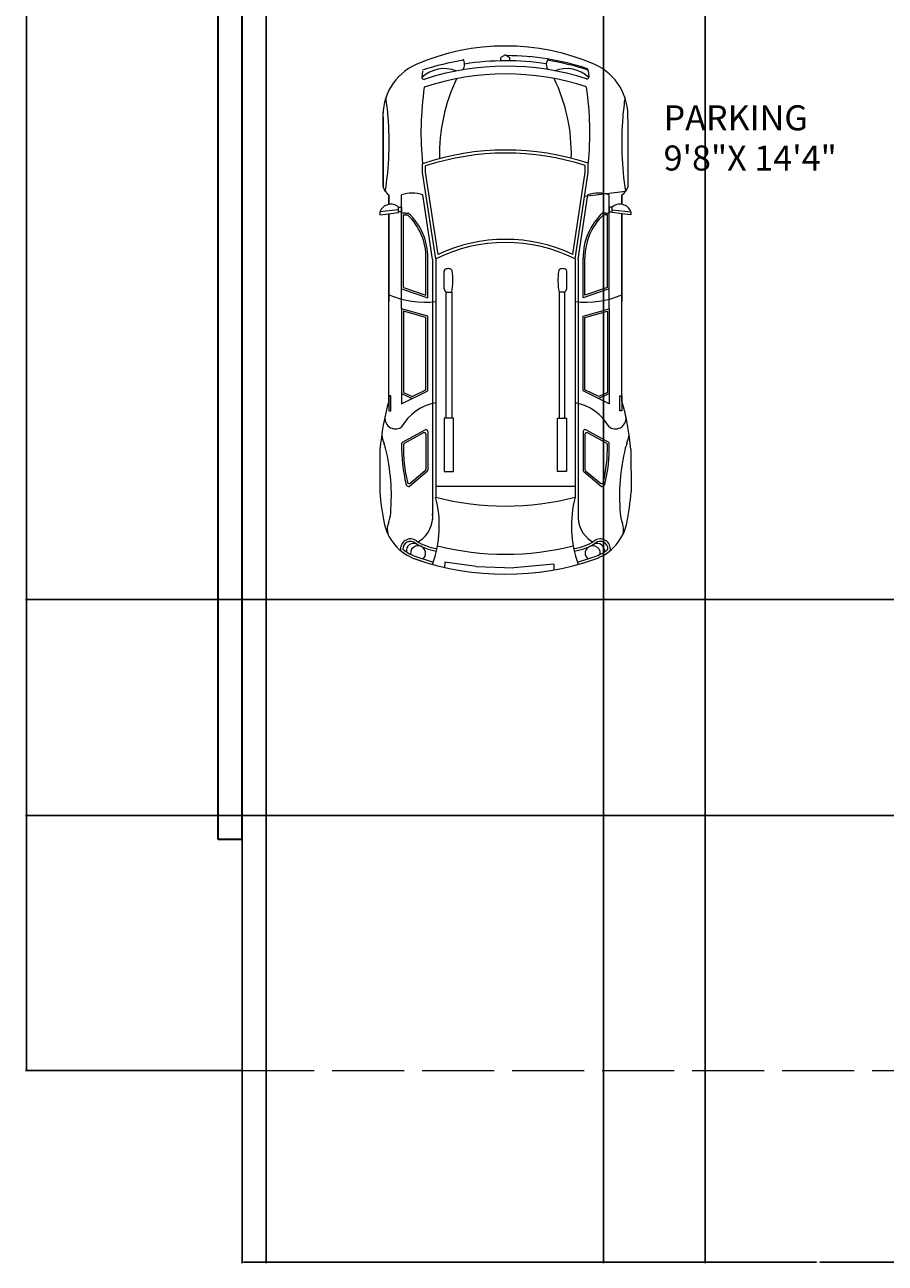
# Model space of a CAD drawing. Units: feet. Extents: x 1993 to 2298, y 2938 to 3641.
# Tile 1 of 11: x 1993 to 2137, y 2938 to 3144. Entities that reach past the tile are written whole.
import ezdxf

# ---------------------------------------------------------------- set-up
doc = ezdxf.new("R2010")
doc.units = ezdxf.units.FT
doc.linetypes.add('ACAD_ISO02W100', pattern=[15, 12, -3])
for name, color, linetype, lineweight in [('A-ANNO-DIMS', 2, 'Continuous', 18), ('A-AREA-IDEN', 7, 'Continuous', 18), ('A-EQPM-VEHC', 8, 'Continuous', 13), ('SUNSHADES', 4, 'ACAD_ISO02W100', 13), ('WAL', 7, 'Continuous', 35)]:
    doc.layers.add(name, color=color, linetype=linetype, lineweight=lineweight)
doc.styles.get("Standard").update_dxf_attribs({"font": 'arial.ttf'})
doc.dimstyles.get("Standard").update_dxf_attribs({"dimtxt": 0.18, "dimasz": 0.18, "dimexe": 0.18, "dimexo": 0.0625, "dimgap": 0.09, "dimtad": 0, "dimtih": 1, "dimtoh": 1, "dimdec": 4, "dimzin": 0, "dimdsep": 46, "dimtxsty": 'Standard', "dimcen": 0.09, "dimadec": 0, "dimazin": 0, "dimtfac": 1, "dimtdec": 4, "dimtofl": 0, "dimtmove": 0, "dimatfit": 3, "dimfxl": 1, "dimtolj": 1, "dimtzin": 0, "dimarcsym": 0})

# ---------------------------------------------------------------- blocks, each defined once
blk = doc.blocks.new('*D56')
at = {"layer": 'A-ANNO-DIMS', "color": 0, "lineweight": -2, "transparency": 16777216}
for p, q in [((2025.7, 3608.53), (1993.61, 3608.53)), ((1993.79, 3608.35), (1993.79, 3289.45)), ((1993.79, 2970.18), (1993.79, 3289.08)), ((2029.7, 2970), (1993.61, 2970))]:
    blk.add_line(p, q, dxfattribs=at)
at = {"layer": 'A-ANNO-DIMS', "color": 0, "transparency": 16777216}
for points in [[(1993.76, 3608.35), (1993.82, 3608.35), (1993.79, 3608.53)], [(1993.76, 2970.18), (1993.82, 2970.18), (1993.79, 2970)]]:
    blk.add_solid(points, dxfattribs=at)
at = {"layer": 'Defpoints', "color": 0, "transparency": 16777216}
for p in [(1993.79, 3608.53), (2025.76, 3608.53), (2029.76, 2970)]:
    blk.add_point(p, dxfattribs=at)
at = {"layer": 'A-ANNO-DIMS', "color": 0, "transparency": 16777216, "insert": (1993.79, 3289.27), "char_height": 0.18, "attachment_point": 5}
blk.add_mtext('\\A1;638.5', dxfattribs=at)
blk = doc.blocks.new('*D57')
at = {"layer": 'A-ANNO-DIMS', "color": 0, "lineweight": -2, "transparency": 16777216}
for p, q in [((2029.76, 2969.94), (2029.76, 2937.86)), ((2221.76, 2969.94), (2221.76, 2937.86)), ((2029.94, 2938.03), (2125.48, 2938.03)), ((2221.58, 2938.03), (2126.04, 2938.03))]:
    blk.add_line(p, q, dxfattribs=at)
at = {"layer": 'A-ANNO-DIMS', "color": 0, "transparency": 16777216}
for points in [[(2029.94, 2938.07), (2029.94, 2938.01), (2029.76, 2938.03)], [(2221.58, 2938.07), (2221.58, 2938.01), (2221.76, 2938.03)]]:
    blk.add_solid(points, dxfattribs=at)
at = {"layer": 'Defpoints', "color": 0, "transparency": 16777216}
for p in [(2029.76, 2970), (2221.76, 2970), (2221.76, 2938.03)]:
    blk.add_point(p, dxfattribs=at)
at = {"layer": 'A-ANNO-DIMS', "color": 0, "transparency": 16777216, "insert": (2125.76, 2938.03), "char_height": 0.18, "attachment_point": 5}
blk.add_mtext('\\A1;192', dxfattribs=at)
blk = doc.blocks.new('*D58')
at = {"layer": 'A-ANNO-DIMS', "color": 0, "lineweight": -2, "transparency": 16777216}
for p, q in [((2139.94, 3048.53), (1993.61, 3048.53)), ((1993.79, 3048.35), (1993.79, 3030.72)), ((1993.79, 3012.71), (1993.79, 3030.35)), ((2139.94, 3012.53), (1993.61, 3012.53))]:
    blk.add_line(p, q, dxfattribs=at)
at = {"layer": 'A-ANNO-DIMS', "color": 0, "transparency": 16777216}
for points in [[(1993.76, 3048.35), (1993.82, 3048.35), (1993.79, 3048.53)], [(1993.76, 3012.71), (1993.82, 3012.71), (1993.79, 3012.53)]]:
    blk.add_solid(points, dxfattribs=at)
at = {"layer": 'Defpoints', "color": 0, "transparency": 16777216}
for p in [(1993.79, 3048.53), (2140, 3048.53), (2140, 3012.53)]:
    blk.add_point(p, dxfattribs=at)
at = {"layer": 'A-ANNO-DIMS', "color": 0, "transparency": 16777216, "insert": (1993.79, 3030.53), "char_height": 0.18, "attachment_point": 5}
blk.add_mtext('\\A1;36', dxfattribs=at)
blk = doc.blocks.new('*D67')
at = {"layer": 'A-ANNO-DIMS', "color": 0, "lineweight": -2, "transparency": 16777216}
for p, q in [((2033.76, 3428.47), (2033.76, 2937.86)), ((2106.96, 3428.47), (2106.96, 2937.86)), ((2033.94, 2938.03), (2070.03, 2938.03)), ((2106.78, 2938.03), (2070.68, 2938.03))]:
    blk.add_line(p, q, dxfattribs=at)
at = {"layer": 'A-ANNO-DIMS', "color": 0, "transparency": 16777216}
for points in [[(2033.94, 2938.07), (2033.94, 2938.01), (2033.76, 2938.03)], [(2106.78, 2938.07), (2106.78, 2938.01), (2106.96, 2938.03)]]:
    blk.add_solid(points, dxfattribs=at)
at = {"layer": 'Defpoints', "color": 0, "transparency": 16777216}
for p in [(2033.76, 3428.53), (2106.96, 3428.53), (2106.96, 2938.03)]:
    blk.add_point(p, dxfattribs=at)
at = {"layer": 'A-ANNO-DIMS', "color": 0, "transparency": 16777216, "insert": (2070.36, 2938.03), "char_height": 0.18, "attachment_point": 5}
blk.add_mtext('\\A1;73.2', dxfattribs=at)
blk = doc.blocks.new('*D71')
at = {"layer": 'A-ANNO-DIMS', "color": 0, "lineweight": -2, "transparency": 16777216}
for p, q in [((2029.76, 3159.94), (2029.76, 2937.86)), ((2090, 3159.94), (2090, 2937.86)), ((2029.94, 2938.03), (2059.49, 2938.03)), ((2089.82, 2938.03), (2060.27, 2938.03))]:
    blk.add_line(p, q, dxfattribs=at)
at = {"layer": 'A-ANNO-DIMS', "color": 0, "transparency": 16777216}
for points in [[(2029.94, 2938.07), (2029.94, 2938.01), (2029.76, 2938.03)], [(2089.82, 2938.07), (2089.82, 2938.01), (2090, 2938.03)]]:
    blk.add_solid(points, dxfattribs=at)
at = {"layer": 'Defpoints', "color": 0, "transparency": 16777216}
for p in [(2029.76, 3160), (2090, 3160), (2090, 2938.03)]:
    blk.add_point(p, dxfattribs=at)
at = {"layer": 'A-ANNO-DIMS', "color": 0, "transparency": 16777216, "insert": (2059.88, 2938.03), "char_height": 0.18, "attachment_point": 5}
blk.add_mtext('\\A1;60.24', dxfattribs=at)
blk = doc.blocks.new('*D75')
at = {"layer": 'A-ANNO-DIMS', "color": 0, "lineweight": -2, "transparency": 16777216}
for p, q in [((2029.76, 3008.6), (2029.76, 3640.68)), ((2029.94, 3640.5), (2084.42, 3640.5)), ((2139.82, 3640.5), (2085.33, 3640.5)), ((2140, 3008.6), (2140, 3640.68))]:
    blk.add_line(p, q, dxfattribs=at)
at = {"layer": 'A-ANNO-DIMS', "color": 0, "transparency": 16777216}
for points in [[(2029.94, 3640.53), (2029.94, 3640.47), (2029.76, 3640.5)], [(2139.82, 3640.53), (2139.82, 3640.47), (2140, 3640.5)]]:
    blk.add_solid(points, dxfattribs=at)
at = {"layer": 'Defpoints', "color": 0, "transparency": 16777216}
for p in [(2140, 3640.5), (2029.76, 3008.53), (2140, 3008.53)]:
    blk.add_point(p, dxfattribs=at)
at = {"layer": 'A-ANNO-DIMS', "color": 0, "transparency": 16777216, "insert": (2084.88, 3640.5), "char_height": 0.18, "attachment_point": 5}
blk.add_mtext('\\A1;110.24', dxfattribs=at)

msp = doc.modelspace()

# ---------------------------------------------------------------- linework, layer by layer
at = {"layer": 'A-EQPM-VEHC'}
for p, q in [((2073.6255, 3139.3497), (2072.864, 3138.9029)), ((2073.6255, 3139.3497), (2074.3869, 3138.9029)), ((2072.864, 3138.3636), (2072.864, 3138.9029)), ((2074.3869, 3138.3636), (2074.3869, 3138.9029)), ((2059.8108, 3136.6444), (2059.7046, 3135.5559)), ((2087.4504, 3136.7145), (2087.5565, 3135.6261)), ((2053.2228, 3117.2778), (2053.2228, 3129.8147)), ((2053.2228, 3128.6448), (2053.2228, 3117.2778)), ((2053.2228, 3128.6448), (2053.2228, 3117.2778)), ((2094.0404, 3128.6448), (2094.0404, 3117.2778)), ((2059.8128, 3119.7356), (2059.8128, 3121.1988)), ((2060.323, 3119.7741), (2060.323, 3120.8311)), ((2086.9402, 3119.7741), (2086.9402, 3120.9002)), ((2087.4504, 3119.7356), (2087.4504, 3121.2699)), ((2062.0034, 3105.3255), (2059.8128, 3119.7356)), ((2062.4037, 3106.0867), (2060.323, 3119.7741)), ((2084.8595, 3106.0867), (2086.9402, 3119.7741)), ((2085.2598, 3105.3255), (2087.4504, 3119.7356)), ((2093.6618, 3116.5742), (2086.843, 3115.7403)), ((2054.2029, 3114.4228), (2054.2029, 3115.9916)), ((2054.2029, 3115.9916), (2054.2029, 3114.4228)), ((2056.3197, 3097.002), (2056.3197, 3115.9891)), ((2056.3197, 3113.9736), (2056.3197, 3115.9891)), ((2061.4931, 3105.287), (2059.8663, 3115.9891)), ((2085.7701, 3105.287), (2087.3969, 3115.9891)), ((2090.9435, 3097.002), (2090.9435, 3115.9891)), ((2090.9435, 3113.9736), (2090.9435, 3115.9891)), ((2093.0603, 3114.4228), (2093.0603, 3115.9916)), ((2093.0603, 3115.9916), (2093.0603, 3114.4228)), ((2053.7156, 3113.3013), (2052.707, 3113.1926)), ((2052.707, 3113.1926), (2052.7076, 3112.6658)), ((2052.7076, 3112.6658), (2053.7156, 3112.8015)), ((2055.8106, 3113.527), (2053.7156, 3113.3013)), ((2053.7156, 3112.8015), (2055.8106, 3113.0836)), ((2054.2029, 3081.6364), (2054.2029, 3112.8671)), ((2054.2029, 3112.8671), (2054.2029, 3098.2087)), ((2055.8106, 3113.0836), (2055.8106, 3113.2072)), ((2056.9702, 3112.9808), (2056.3197, 3112.9808)), ((2056.6258, 3100.5765), (2056.6258, 3112.6747)), ((2056.771, 3112.6747), (2056.6258, 3112.6747)), ((2056.6258, 3112.6747), (2057.3067, 3112.6747)), ((2056.9702, 3112.9808), (2057.4267, 3112.9808)), ((2090.293, 3112.9808), (2089.8365, 3112.9808)), ((2090.6374, 3112.6747), (2089.9565, 3112.6747)), ((2090.293, 3112.9808), (2090.9435, 3112.9808)), ((2090.4922, 3112.6747), (2090.6374, 3112.6747)), ((2090.6374, 3100.5765), (2090.6374, 3112.6747)), ((2091.4526, 3113.527), (2093.5476, 3113.3013)), ((2091.4526, 3113.0836), (2091.4526, 3113.2072)), ((2093.5476, 3112.8015), (2091.4526, 3113.0836)), ((2093.0603, 3081.6364), (2093.0603, 3112.8671)), ((2093.0603, 3112.8671), (2093.0603, 3098.2087)), ((2093.5476, 3113.3013), (2094.5562, 3113.1926)), ((2094.5556, 3112.6658), (2093.5476, 3112.8015)), ((2094.5562, 3113.1926), (2094.5556, 3112.6658)), ((2060.3766, 3099.2754), (2060.3766, 3105.4613)), ((2060.3766, 3102.6251), (2060.3766, 3104.5322)), ((2060.6827, 3104.5969), (2060.6827, 3105.4613)), ((2060.6827, 3102.6251), (2060.6827, 3104.5969)), ((2061.4809, 3105.287), (2061.4809, 3061.8298)), ((2061.4931, 3105.287), (2061.4931, 3061.9649)), ((2062.0034, 3105.3255), (2062.0034, 3065.5612)), ((2085.2598, 3105.3255), (2085.2598, 3065.6082)), ((2085.7701, 3105.287), (2085.7701, 3061.8298)), ((2086.5805, 3104.5969), (2086.5805, 3105.4613)), ((2086.5805, 3102.6251), (2086.5805, 3104.5969)), ((2086.8866, 3099.2754), (2086.8866, 3105.4613)), ((2086.8866, 3102.6251), (2086.8866, 3104.5322)), ((2060.3766, 3099.2754), (2060.3766, 3102.6251)), ((2060.6827, 3098.8452), (2060.6827, 3102.6251)), ((2063.4098, 3100.3569), (2063.4098, 3103.2792)), ((2083.8411, 3100.3569), (2083.8411, 3103.2792)), ((2086.5805, 3098.8452), (2086.5805, 3102.6251)), ((2086.8866, 3099.2754), (2086.8866, 3102.6251)), ((2056.3197, 3100.3587), (2060.6827, 3098.8452)), ((2056.6258, 3100.5765), (2060.3766, 3099.2754)), ((2090.9435, 3100.3587), (2086.5805, 3098.8452)), ((2090.6374, 3100.5765), (2086.8866, 3099.2754)), ((2056.3197, 3097.002), (2056.3197, 3081.1516)), ((2060.6827, 3095.7692), (2056.3197, 3097.002)), ((2056.6258, 3096.5974), (2056.6258, 3083.0672)), ((2060.3766, 3095.5376), (2056.6258, 3096.5974)), ((2060.6827, 3083.3358), (2060.6827, 3095.7692)), ((2086.5805, 3095.7692), (2090.9435, 3097.002)), ((2086.5805, 3083.3358), (2086.5805, 3095.7692)), ((2086.8866, 3095.5376), (2090.6374, 3096.5974)), ((2090.6374, 3096.5974), (2090.6374, 3083.0672)), ((2090.9435, 3097.002), (2090.9435, 3081.1516)), ((2060.3766, 3083.5249), (2060.3766, 3095.5376)), ((2086.8866, 3083.5249), (2086.8866, 3095.5376)), ((2058.0804, 3082.3754), (2060.3766, 3083.5249)), ((2089.1828, 3082.3754), (2086.8866, 3083.5249)), ((2056.3197, 3081.1516), (2060.6827, 3083.3358)), ((2056.3197, 3082.8738), (2058.0838, 3082.0348)), ((2056.6258, 3083.0672), (2058.0804, 3082.3754)), ((2090.9435, 3081.1516), (2086.5805, 3083.3358)), ((2090.9435, 3082.8738), (2089.1794, 3082.0348)), ((2090.6374, 3083.0672), (2089.1828, 3082.3754)), ((2056.4738, 3074.7613), (2060.2287, 3076.8322)), ((2056.777, 3074.5789), (2059.9226, 3076.3137)), ((2060.3766, 3076.0457), (2060.3766, 3070.2522)), ((2060.6827, 3076.5641), (2060.6827, 3070.1104)), ((2086.5805, 3076.5641), (2086.5805, 3070.1104)), ((2086.8866, 3076.0457), (2086.8866, 3070.2522)), ((2090.7894, 3074.7613), (2087.0345, 3076.8322)), ((2090.4862, 3074.5789), (2087.3406, 3076.3137)), ((2052.715, 3073.5228), (2052.6794, 3066.5123)), ((2094.5482, 3073.5228), (2094.5838, 3066.5123)), ((2060.5745, 3069.8769), (2057.6245, 3067.3762)), ((2060.2684, 3070.0187), (2057.797, 3067.9237)), ((2086.6887, 3069.8769), (2089.6387, 3067.3762)), ((2086.9948, 3070.0187), (2089.4662, 3067.9237)), ((2085.2598, 3067.3782), (2062.0034, 3067.3782)), ((2063.5088, 3054.7422), (2063.4967, 3053.8931)), ((2068.7637, 3054.0321), (2063.5088, 3054.7422)), ((2061.4809, 3054.3994), (2061.4809, 3054.3961)), ((2061.4931, 3054.43), (2061.4931, 3054.3961)), ((2068.7637, 3054.0321), (2075.031, 3053.7898)), ((2081.6726, 3054.4006), (2075.031, 3053.7898)), ((2081.6726, 3054.4006), (2081.6784, 3053.4697)), ((2085.7701, 3054.3994), (2085.7701, 3054.3961))]:
    msp.add_line(p, q, dxfattribs=at)
for points in [[(2056.3197, 3113.9736), (2056.3197, 3113.2072), (2055.8106, 3113.2072), (2055.8106, 3113.9736)], [(2090.9435, 3113.9736), (2090.9435, 3113.2072), (2091.4526, 3113.2072), (2091.4526, 3113.9736)], [(2063.7437, 3078.7492), (2063.7437, 3099.7661), (2064.6874, 3099.7661), (2064.6874, 3078.7492)], [(2083.5072, 3078.7492), (2083.5072, 3099.7661), (2082.5636, 3099.7661), (2082.5636, 3078.7492)], [(2054.2029, 3082.4766), (2054.2029, 3080.0221), (2054.5357, 3080.0221), (2054.5357, 3082.4766)], [(2093.0603, 3082.4766), (2093.0603, 3080.0221), (2092.7275, 3080.0221), (2092.7275, 3082.4766)], [(2063.4381, 3078.7492), (2063.4381, 3069.8666), (2064.9651, 3069.8666), (2064.9651, 3078.7492)], [(2083.8129, 3078.7492), (2083.8129, 3069.8666), (2082.2859, 3069.8666), (2082.2859, 3078.7492)]]:
    msp.add_lwpolyline(points, close=True, dxfattribs=at)
for centre, radius, start, end in [((2073.6316, 3103.2534), 37.5749, 66.630379, 113.369621), ((2073.7376, 3095.7735), 43.4568, 71.997404, 89.879209), ((2062.5318, 3129.2298), 9.3273, 114.073482, 183.59562), ((2062.5318, 3129.2298), 9.3273, 114.073482, 183.59562), ((2063.4264, 3131.7153), 5.3481, 67.925574, 134.099571), ((2073.5134, 3095.7735), 43.2527, 99.138951, 108.471967), ((2073.7376, 3094.0149), 43.4568, 71.997404, 108.299537), ((2065.3709, 3137.7851), 1.4594, 320.933681, 37.050913), ((2073.7376, 3094.9141), 43.4568, 81.135241, 99.146235), ((2079.6361, 3139.0906), 1.9662, 181.126018, 181.925536), ((2081.8923, 3137.7851), 1.4594, 142.949087, 217.050913), ((2073.7376, 3095.7735), 43.2527, 71.528033, 80.861049), ((2083.8245, 3131.7153), 5.3481, 45.900429, 112.074426), ((2087.0422, 3136.7145), 0.4082, 0, 71.997404), ((2087.0422, 3136.7145), 0.4082, 0, 71.997404), ((2084.7314, 3129.2298), 9.3273, 356.40438, 65.926518), ((2060.0928, 3135.6821), 0.4082, 198.002596, 270), ((2073.7376, 3092.7129), 43.4568, 71.997404, 108.299537), ((2091.484, 3122.8842), 28.8394, 154.32269, 181.54108), ((2055.7792, 3122.8842), 28.8394, 358.45892, 25.775323), ((2087.1683, 3135.7523), 0.4082, 270, 341.997404), ((2111.6717, 3126.4516), 52.1243, 171.704533, 185.783782), ((2035.5792, 3126.4516), 52.1243, 354.216218, 8.295467), ((2003.0554, 3124.7045), 51.1957, 4.81443, 8.440878), ((2144.2078, 3124.7045), 51.1957, 171.559122, 175.18557), ((2144.2078, 3124.7045), 51.1957, 171.559122, 171.624919), ((2003.0554, 3124.7045), 51.1957, 350.862268, 4.81443), ((2144.2078, 3124.7045), 51.1957, 175.18557, 189.137732), ((2073.7376, 3080.0334), 43.4568, 71.605988, 108.68883), ((2073.7376, 3080.0334), 42.9465, 72.096283, 108.201197), ((2055.7359, 3118.1764), 2.669, 199.674985, 234.980034), ((2091.5273, 3118.1764), 2.669, 305.019966, 340.325015), ((2054.5318, 3112.4983), 1.9524, 49.080952, 159.168526), ((2058.093, 3111.3014), 5.0119, 140.910288, 141.57576), ((2058.093, 3111.3014), 5.0119, 69.279371, 110.720629), ((2089.1702, 3111.3014), 5.0119, 69.279371, 110.720629), ((2092.7314, 3112.4983), 1.9524, 20.831474, 130.919048), ((2089.1702, 3111.3014), 5.0119, 38.42424, 39.089712), ((2050.6599, 3105.5861), 9.7175, 359.286552, 46.842), ((2050.6599, 3105.5861), 10.0236, 359.286552, 47.538618), ((2096.6033, 3105.5861), 10.0236, 132.461382, 180.713448), ((2096.6033, 3105.5861), 9.7175, 133.158, 180.713448), ((2073.6316, 3082.1299), 26.4573, 64.888829, 115.111171), ((2073.6316, 3082.1299), 25.9471, 63.374856, 116.625144), ((2063.818, 3103.2792), 0.4082, 99.76289, 180), ((2064.0344, 3102.0214), 1.6844, 76.115932, 99.76289), ((2064.3407, 3103.2604), 0.4082, 8.618675, 76.115932), ((2054.1329, 3101.7132), 10.7326, 349.547488, 8.618675), ((2093.1181, 3101.7132), 10.7326, 171.381325, 190.452512), ((2082.9103, 3103.2604), 0.4082, 103.884068, 171.381325), ((2083.2165, 3102.0214), 1.6844, 80.23711, 103.884068), ((2083.4329, 3103.2792), 0.4082, 0, 80.23711), ((2064.4818, 3100.573), 1.0936, 191.396908, 227.548239), ((2082.7691, 3100.573), 1.0936, 312.451761, 348.603092), ((2060.2931, 3113.7813), 15.6663, 247.12347, 276.267274), ((2073.6316, 3082.1299), 25.9471, 138.443699, 138.484815), ((2086.9701, 3113.7813), 15.6663, 263.732726, 292.87653), ((2095.8876, 3069.7986), 43.3329, 164.146361, 175.069713), ((2063.6007, 3073.0815), 8.4285, 101.138754, 149.775439), ((2083.6625, 3073.0815), 8.4285, 30.224561, 78.861246), ((2051.3756, 3069.7986), 43.3329, 4.930287, 15.853639), ((2055.3057, 3078.7586), 1.7763, 164.377378, 302.119003), ((2111.6717, 3126.4516), 52.1243, 240.109305, 240.203455), ((2091.9575, 3078.7586), 1.7763, 237.880997, 15.622622), ((2056.1417, 3077.427), 0.2041, 302.119003, 329.775439), ((2091.1215, 3077.427), 0.2041, 210.224561, 237.880997), ((2059.0076, 3076.8185), 6.0575, 187.596614, 201.790491), ((2060.0704, 3076.0457), 0.3061, 0, 118.876578), ((2060.3766, 3076.5641), 0.3061, 0, 118.876578), ((2086.8866, 3076.5641), 0.3061, 61.123422, 180), ((2087.1928, 3076.0457), 0.3061, 61.123422, 180), ((2088.2556, 3076.8185), 6.0575, 338.209509, 352.403386), ((2047.6977, 3072.2971), 6.1226, 13.816524, 21.790491), ((2021.0595, 3065.746), 33.5546, 355.172787, 13.816524), ((2082.3547, 3073.9831), 26.0442, 178.8643, 193.926241), ((2056.6217, 3074.4933), 0.3061, 118.876578, 178.8643), ((2082.3547, 3073.9831), 25.7381, 179.2616, 193.242697), ((2056.9248, 3074.3109), 0.3061, 118.876578, 179.2616), ((2064.9085, 3073.9831), 25.7381, 346.757303, 0.7384), ((2064.9085, 3073.9831), 26.0442, 346.073759, 1.1357), ((2090.3384, 3074.3109), 0.3061, 0.7384, 61.123422), ((2090.6415, 3074.4933), 0.3061, 1.1357, 61.123422), ((2126.2037, 3065.746), 33.5546, 166.183476, 184.827213), ((2099.5655, 3072.2971), 6.1226, 158.209509, 166.183476), ((2060.0704, 3070.2522), 0.3061, 310.287322, 0), ((2060.3766, 3070.1104), 0.3061, 310.287322, 0), ((2086.8866, 3070.1104), 0.3061, 180, 229.712678), ((2087.1928, 3070.2522), 0.3061, 180, 229.712678), ((2057.3731, 3067.7887), 0.3061, 193.926241, 223.375537), ((2057.6199, 3068.0218), 0.6456, 223.375537, 270.411485), ((2057.599, 3068.1573), 0.3061, 193.242697, 310.287322), ((2089.6642, 3068.1573), 0.3061, 229.712678, 346.757303), ((2089.6433, 3068.0218), 0.6456, 269.588515, 316.624463), ((2089.8901, 3067.7887), 0.3061, 316.624463, 346.073759), ((2095.8876, 3069.7986), 43.3329, 184.349473, 191.387187), ((2043.6982, 3060.823), 18.9084, 340.12943, 14.659569), ((2073.6316, 3109.861), 45.755, 255.277296, 284.722704), ((2103.5527, 3060.823), 18.9084, 165.340431, 199.87057), ((2051.3756, 3069.7986), 43.3329, 348.612813, 355.650527), ((2048.3942, 3063.4375), 6.1226, 339.290067, 355.172787), ((2056.7032, 3062.3307), 4.8039, 302.339468, 5.986075), ((2090.5477, 3062.3307), 4.8039, 174.013925, 237.660532), ((2098.869, 3063.4375), 6.1226, 184.827213, 200.709933), ((2061.3741, 3062.9704), 8.1635, 190.173705, 250.989219), ((2061.3741, 3062.9704), 8.1635, 190.173705, 250.989219), ((2061.3863, 3062.9704), 8.1635, 190.173705, 250.989219), ((2056.955, 3060.201), 3.0296, 159.290067, 194.272559), ((2085.8769, 3062.9704), 8.1635, 289.010781, 349.826295), ((2090.3082, 3060.201), 3.0296, 345.727441, 20.709933), ((2057.7959, 3056.9638), 1.6695, 52.710583, 189.111116), ((2089.4551, 3056.9638), 1.6695, 350.888884, 127.289417), ((2057.7959, 3056.9638), 1.2614, 52.710583, 182.470955), ((2057.7959, 3056.9638), 1.2614, 51.971171, 182.470955), ((2061.3741, 3062.9704), 7.7553, 231.399964, 250.989219), ((2058.3639, 3056.6264), 1.2614, 67.953656, 186.080028), ((2059.0618, 3056.2454), 1.2614, 310.991042, 187.443097), ((2063.5473, 3065.7844), 9.2739, 237.56214, 261.230167), ((2059.0546, 3058.6169), 0.4082, 232.710583, 302.339468), ((2059.0546, 3058.6169), 0.4082, 232.710583, 302.339468), ((2059.0546, 3058.6169), 0.4082, 232.710583, 302.339468), ((2059.0546, 3058.6169), 0.4082, 232.710583, 302.339468), ((2063.5473, 3065.7844), 8.8657, 237.680475, 261.389534), ((2058.3639, 3056.6264), 1.2614, 52.710583, 53.027005), ((2073.6194, 3101.8442), 45.755, 255.694664, 284.320469), ((2073.6316, 3101.8442), 45.755, 255.679531, 284.305336), ((2083.7036, 3065.7844), 8.8657, 278.610466, 302.319525), ((2083.7036, 3065.7844), 9.2739, 278.769833, 302.43786), ((2088.1892, 3056.2454), 1.2614, 352.556903, 229.008958), ((2088.1963, 3058.6169), 0.4082, 237.660532, 307.289417), ((2088.1963, 3058.6169), 0.4082, 237.660532, 307.289417), ((2088.1963, 3058.6169), 0.4082, 237.660532, 307.289417), ((2088.1963, 3058.6169), 0.4082, 237.660532, 307.289417), ((2088.887, 3056.6264), 1.2614, 126.972995, 127.289417), ((2085.8769, 3062.9704), 7.7553, 289.010781, 308.600036), ((2088.887, 3056.6264), 1.2614, 353.919972, 112.046344), ((2089.4551, 3056.9638), 1.2614, 357.529045, 128.028829), ((2089.4551, 3056.9638), 1.2614, 357.529045, 127.289417), ((2073.6194, 3098.5116), 45.755, 250.989219, 289.010781), ((2073.6194, 3098.5116), 45.755, 250.989219, 289.010781), ((2073.6316, 3098.5116), 45.755, 250.989219, 289.010781), ((2073.6316, 3098.5116), 45.755, 250.989219, 289.010781), ((2073.6194, 3098.5116), 45.3469, 250.989219, 254.650531), ((2073.6316, 3098.5116), 45.3469, 285.349469, 289.010781)]:
    msp.add_arc(centre, radius, start, end, dxfattribs=at)
at = {"layer": 'SUNSHADES'}
for p, q in [((2029.7583, 3008.5338), (2029.7583, 2970)), ((2029.7583, 2970), (2221.7583, 2970))]:
    msp.add_line(p, q, dxfattribs=at)
at = {"layer": 'WAL'}
for p, q in [((2025.7583, 3008.5338), (2025.7583, 3608.5338)), ((2029.7583, 3008.5338), (2029.7583, 3184.5338)), ((2029.7583, 3008.5338), (2025.7583, 3008.5338))]:
    msp.add_line(p, q, dxfattribs=at)

# ---------------------------------------------------------------- texts
at = {"layer": 'A-AREA-IDEN'}
for s, height, p in [('PARKING', 4.17051, (2100, 3126.7707)), ('9\'8"X 14\'4"', 4.170506, (2100, 3120.0711))]:
    msp.add_text(s, height=height, dxfattribs=at).set_placement(p)

# ---------------------------------------------------------------- dimensions: what is measured, and where the dimension line sits
at = {"layer": 'A-ANNO-DIMS'}
for base, p1, p2, override, picture, middle in [((2140, 3640.4988), (2029.7583, 3008.5338), (2140, 3008.5338), {"dimdec": 2, "dimlfac": 1, "dimrnd": 0, "dimzin": 0, "dimdsep": 46, "dimlunit": 2}, '*D75', (2084.8792, 3640.4988)), ((2106.9556, 2938.035), (2033.7583, 3428.5338), (2106.9556, 3428.5338), {"dimdec": 1, "dimlfac": 1, "dimrnd": 0, "dimzin": 0, "dimdsep": 46, "dimlunit": 2}, '*D67', (2070.357, 2938.035)), ((2090, 2938.035), (2029.7583, 3160), (2090, 3160), {"dimdec": 2, "dimlfac": 1, "dimrnd": 0, "dimzin": 0, "dimdsep": 46, "dimlunit": 2}, '*D71', (2059.8792, 2938.035)), ((2221.7583, 2938.035), (2029.7583, 2970), (2221.7583, 2970), {"dimdec": 0, "dimlfac": 1, "dimrnd": 0, "dimzin": 0, "dimdsep": 46, "dimlunit": 2}, '*D57', (2125.7583, 2938.035))]:
    dim = msp.add_linear_dim(base=base, p1=p1, p2=p2, dimstyle='Standard', override=override, dxfattribs=at)
    dim.commit()
    dim.dimension.update_dxf_attribs({"geometry": picture, "text_midpoint": middle})
for base, p1, p2, override, picture, middle in [((1993.7933, 3608.5338), (2029.7583, 2970), (2025.7583, 3608.5338), {"dimdec": 1, "dimlfac": 1, "dimrnd": 0, "dimzin": 0, "dimdsep": 46, "dimlunit": 2}, '*D56', (1993.7933, 3289.2669)), ((1993.7933, 3048.5338), (2140, 3012.5338), (2140, 3048.5338), {"dimdec": 0, "dimlfac": 1, "dimrnd": 0, "dimzin": 0, "dimdsep": 46, "dimlunit": 2}, '*D58', (1993.7933, 3030.5338))]:
    dim = msp.add_linear_dim(base=base, p1=p1, p2=p2, angle=90, dimstyle='Standard', override=override, dxfattribs=at)
    dim.commit()
    dim.dimension.update_dxf_attribs({"geometry": picture, "text_midpoint": middle})

doc.saveas('drawing.dxf')
